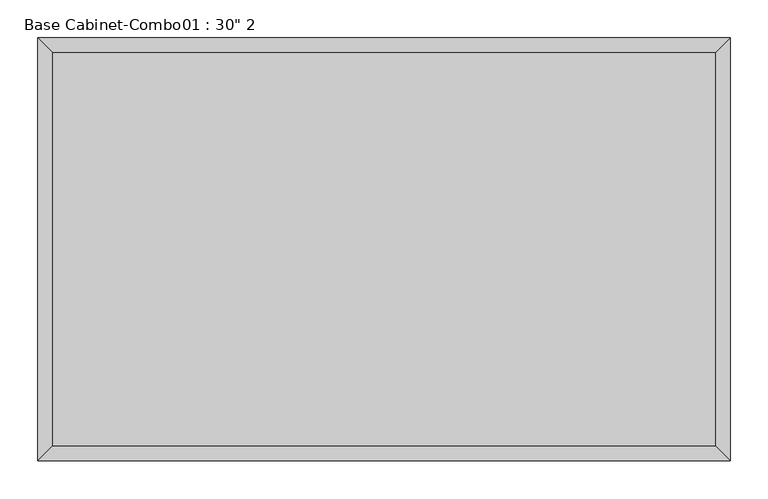
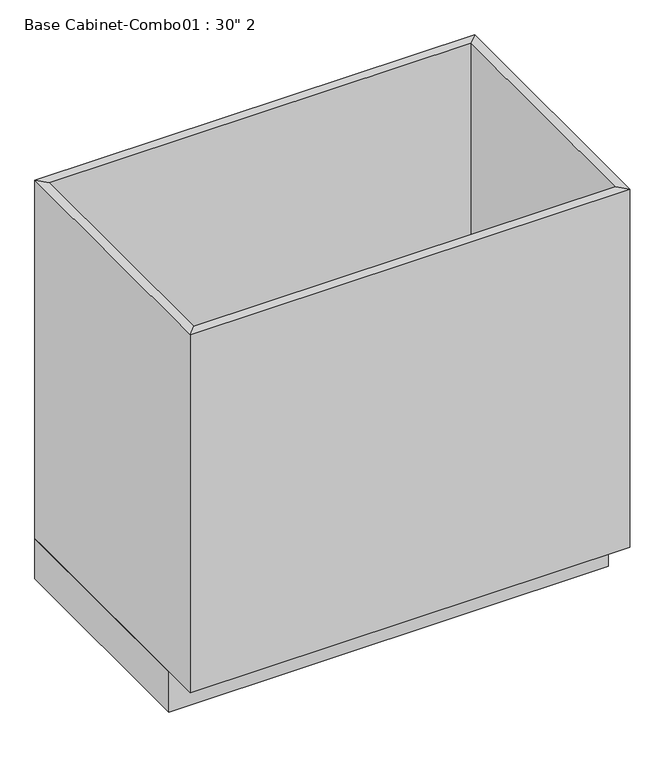
"""IFC4 building model written with IfcOpenShell, lengths in millimetres: furniture geometry."""

from ifc_helpers import new_model, si_unit, frame, origin, origin_with_axes, place, context, project, spatial, polyline, outline, extrude, faceted_brep, source, transform, mapped, element, save


def furniture_bf8a676d(model_context):
    return source(origin(), model_context, "Body", "SolidModel", [
        extrude(outline(polyline([(475.9377049, 0.0), (475.9377049, -482.6), (-438.4622951, -482.6), (-438.4622951, 0.0), (475.9377049, 0.0)])), origin_with_axes(), (0.0, 0.0, 1.0), 88.9),
        faceted_brep([(456.8877049, -539.75, 876.3), (456.8877049, -539.75, 88.9), (-419.4122951, -539.75, 88.9), (-419.4122951, -539.75, 876.3), (475.9377049, -558.8, 876.3), (-438.4622951, -558.8, 876.3), (475.9377049, -558.8, 88.9), (-438.4622951, -558.8, 88.9), (-419.4122951, -19.05, 88.9), (-419.4122951, -19.05, 876.3), (-438.4622951, 0.0, 876.3), (-438.4622951, 0.0, 88.9), (456.8877049, -19.05, 88.9), (456.8877049, -19.05, 876.3), (475.9377049, 0.0, 876.3), (475.9377049, 0.0, 88.9)], [[[0, 1, 2, 3]], [[4, 0, 3, 5]], [[6, 4, 5, 7]], [[1, 6, 7, 2]], [[3, 2, 8, 9]], [[5, 3, 9, 10]], [[7, 5, 10, 11]], [[2, 7, 11, 8]], [[9, 8, 12, 13]], [[10, 9, 13, 14]], [[11, 10, 14, 15]], [[8, 11, 15, 12]], [[13, 12, 1, 0]], [[14, 13, 0, 4]], [[15, 14, 4, 6]], [[12, 15, 6, 1]]]),
        extrude(outline(polyline([(456.8877049, -19.05), (456.8877049, -539.75), (-419.4122951, -539.75), (-419.4122951, -19.05), (456.8877049, -19.05)])), frame((0.0, 0.0, 88.9), z_axis=(0.0, 0.0, 1.0), x_axis=(1.0, 0.0, 0.0)), (0.0, 0.0, 1.0), 19.05),
    ])


if __name__ == "__main__":
    model = new_model("IFC4")
    model_context = context("Model", 3, world=origin())
    ifc_project = project(units=[si_unit("LENGTHUNIT", "METRE", prefix="MILLI")], contexts=[model_context])
    site = spatial("IfcSite", under=ifc_project)
    building = spatial("IfcBuilding", under=site)
    placement = place(None, origin())
    furniture_shape = furniture_bf8a676d(model_context)
    element("IfcFurniture", 1, ObjectType="Base Cabinet-Combo01 : 30\" 2", at=placement, inside=building, context=model_context, shape_type="MappedRepresentation", body=[
        mapped(furniture_shape, transform((0.0, 0.0, 0.0), x_axis=(1.0, 0.0, 0.0), y_axis=(0.0, 1.0, 0.0), z_axis=(0.0, 0.0, 1.0))),
    ])
    save(model, "model.ifc")

# Revit data of these elements
# Type "Base Cabinet-Combo01 : 30\" 2"
#   Depth = 1' - 10"
#   Height = 2' - 10 1/2"
#   Toe Depth = 0' - 3"
#   Toe Height = 0' - 3 1/2"
#   Width = 3' - 0"
#   Default Elevation = 0
# Element 1 (IfcFurniture, "Base Cabinet-Combo01 : 30\" 2")
#   Materials on its faces: "Cabinet"
# Materials
#   "Cabinet": colour RGB 204 122 2, transparency 0
